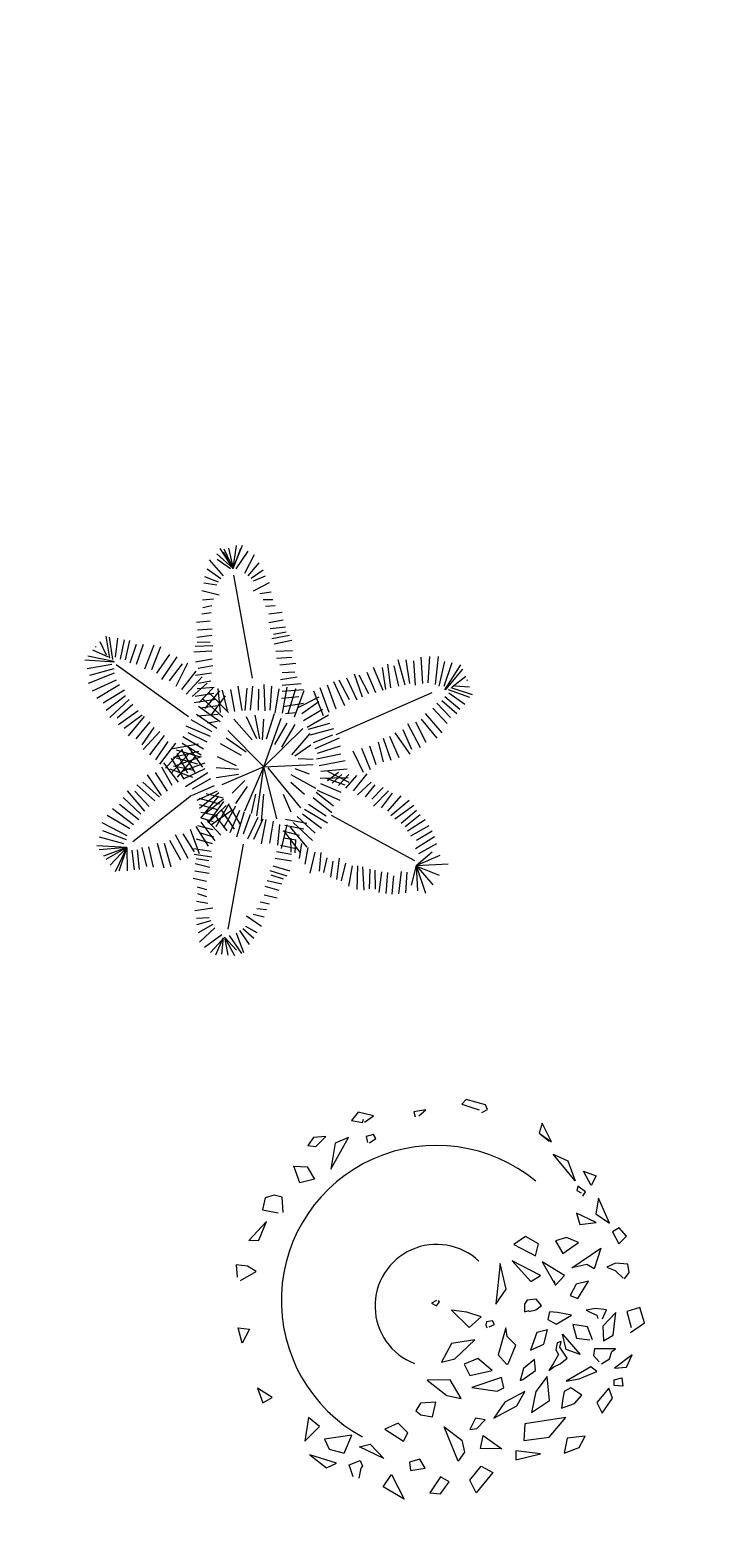
# Model space of a CAD drawing. Units: inches. Extents: x 8049 to 8459, y 820 to 1350.
# Tile 12 of 25: x 8157 to 8170, y 877 to 906. Entities that reach past the tile are written whole.
import ezdxf

# ---------------------------------------------------------------- set-up
doc = ezdxf.new("R2010")
doc.units = ezdxf.units.IN
doc.header["$MEASUREMENT"] = 0
doc.layers.add('A-ANNO-DIMS', color=2, linetype='Continuous', lineweight=18)
doc.layers.add('zelen', color=69, linetype='Continuous', lineweight=13)
doc.styles.get("Standard").update_dxf_attribs({"font": 'arial.ttf'})
doc.dimstyles.get("Standard").update_dxf_attribs({"dimtxt": 0.18, "dimasz": 0.18, "dimexe": 0.18, "dimexo": 0.0625, "dimgap": 0.09, "dimtad": 0, "dimtih": 1, "dimtoh": 1, "dimdec": 4, "dimzin": 0, "dimdsep": 46, "dimtxsty": 'Standard', "dimcen": 0.09, "dimadec": 0, "dimazin": 0, "dimtfac": 1, "dimtdec": 4, "dimtofl": 0, "dimtmove": 0, "dimatfit": 3, "dimfxl": 1, "dimtolj": 1, "dimtzin": 0, "dimarcsym": 0})

# ---------------------------------------------------------------- blocks, each defined once
blk = doc.blocks.new('z_86')
for p, q in [((-83.5, 478), (-122.3, 513.6)), ((-83.5, 478), (-114.5, 526.5)), ((-83.5, 478), (-106.5, 517.8)), ((-105.6, 525.2), (-83.5, 478)), ((-94.4, 527.5), (-83.5, 478)), ((-83.5, 478), (-61.2, 534.1)), ((-83.5, 478), (-75.1, 533.5)), ((-83.5, 478), (-65.1, 526.2)), ((-76.2, 477.3), (-47.6, 520.2)), ((-55.2, 467.1), (-32.4, 512)), ((-112.8, 453.1), (-146, 476.4)), ((-106.9, 460.9), (-139.8, 499)), ((-89.5, 477.3), (-121.9, 499.8)), ((-47.6, 461), (-21, 491.6)), ((-40, 454.9), (-11.4, 475.3)), ((-122.8, 438), (-153.5, 443.1)), ((-118.8, 445.3), (-151.4, 458.3)), ((-36.9, 215.2), (-81.5, 462)), ((-34.3, 448.8), (-5.7, 461)), ((-34.3, 424.3), (3.8, 444.7)), ((-117, 414.2), (-158.9, 425)), ((-130.3, 404.7), (-157.2, 402.3)), ((-19.1, 418.2), (7.6, 422.3)), ((-11.4, 403.9), (11.4, 403.9)), ((-135.9, 371.8), (-158.6, 368.3)), ((-134.3, 389), (-156.5, 383.5)), ((-5.7, 387.6), (17.1, 389.6)), ((1.9, 369.2), (34.3, 373.3)), ((-138.9, 352.1), (-171.3, 348.3)), ((-134, 332.3), (-168.8, 330.1)), ((1.9, 348.8), (36.2, 354.9)), ((5.7, 334.5), (41.9, 338.6)), ((13.3, 320.3), (43.8, 326.4)), ((-412.2, 291.3), (-413.8, 289.4)), ((-387.3, 269.9), (-402.1, 302.2)), ((-379.4, 263.2), (-388.4, 316.1)), ((-371.9, 259.8), (-379.8, 313.8)), ((-365.6, 265.3), (-360, 311.4)), ((-353.9, 260.7), (-343.8, 307)), ((-341.4, 258.8), (-331.3, 305.1)), ((-330.6, 251.5), (-315.1, 296.4)), ((-315.3, 248.9), (-298.9, 296.4)), ((-295.6, 237.8), (-272.9, 295.1)), ((-278.5, 236), (-256.7, 290.7)), ((-132.2, 292.8), (-174.8, 290.8)), ((-134.3, 317.5), (-170.4, 312.8)), ((-138.3, 301.8), (-169.4, 300.5)), ((9.5, 310), (51.4, 318.2)), ((15.2, 297.8), (57.1, 306)), ((-368.1, 253.4), (-438.9, 258.6)), ((-370, 255.1), (-431.7, 268)), ((-382.4, 265.8), (-420.1, 282.2)), ((-266.9, 227.1), (-235.2, 271.9)), ((-254.3, 212.2), (-218.1, 265.9)), ((-220.3, 195.8), (-192.1, 251.6)), ((-134.8, 279.6), (-177.4, 277.5)), ((-134.1, 260.9), (-173.4, 253.3)), ((19, 279.5), (59, 281.5)), ((20.9, 263.1), (57.1, 265.2)), ((329.4, 197.9), (312.2, 259.1)), ((340.8, 201.9), (331.3, 259.1)), ((354.1, 197.9), (350.3, 257)), ((371.3, 201.9), (367.5, 265.2)), ((384.6, 204), (388.4, 267.2)), ((401.7, 199.9), (409.4, 267.2)), ((411.2, 195.8), (424.6, 255)), ((422.7, 195.8), (441.7, 252.9)), ((-374.7, 247.6), (-434, 237.7)), ((-368.5, 227.2), (-431.5, 202.4)), ((-369.3, 237.5), (-427.8, 221.6)), ((-190.5, 122.3), (-363.9, 247)), ((-236.4, 208.8), (-204.7, 249.3)), ((-206.8, 187.8), (-172.4, 231.9)), ((-196.1, 176.3), (-158.1, 217.9)), ((-135.5, 226.9), (-173.5, 221.8)), ((-132, 244.6), (-167.7, 237.9)), ((28.5, 246.8), (66.6, 250.9)), ((30.5, 212.1), (70.4, 218.3)), ((34.3, 228.4), (64.7, 230.5)), ((188.5, 216.2), (213.2, 163.2)), ((226.6, 169.3), (207.5, 224.4)), ((241.8, 177.5), (218.9, 222.4)), ((258.9, 179.5), (238, 228.4)), ((276.1, 185.6), (253.2, 240.7)), ((274.2, 240.7), (281.8, 187.7)), ((295.1, 191.7), (287.5, 248.9)), ((314.1, 195.8), (302.7, 244.8)), ((424.7, 187.2), (462.5, 247.4)), ((427.1, 188.2), (467.4, 236.7)), ((442.4, 194.2), (474.5, 219.7)), ((-364.1, 210.1), (-421.7, 183.9)), ((-356, 199.3), (-410.1, 166.3)), ((-344.4, 186.1), (-394.9, 155)), ((-181.7, 171), (-145.6, 203)), ((-129.1, 192.8), (-169.4, 189.2)), ((-136.7, 207.7), (-166.7, 202.4)), ((-164.7, 156.3), (-132.2, 190.7)), ((-150.4, 142.3), (-115.1, 184.7)), ((-94.3, 132.6), (-142, 180.7)), ((-113.5, 132.6), (-119.3, 190.6)), ((-96.8, 137.1), (-108.7, 186)), ((-79.7, 135.1), (-88.7, 187.5)), ((-61.5, 137.1), (-71, 196)), ((-50.7, 191.1), (-55.5, 137.7)), ((-41.6, 138.6), (-35.8, 196)), ((-22.2, 138.2), (-21.9, 188.5)), ((-6.8, 136.7), (-9.4, 200.2)), ((5.2, 138), (9.1, 195.8)), ((17.2, 130.9), (27.2, 189.4)), ((34.3, 197.9), (80, 201.9)), ((34.3, 183.6), (85.7, 187.7)), ((34.8, 130.9), (45.8, 193.4)), ((48.3, 129.9), (66.6, 190.5)), ((64, 121.9), (87, 185.6)), ((133.3, 124.4), (110.4, 183.6)), ((146.6, 132.6), (125.6, 191.7)), ((163.7, 140.7), (142.8, 197.9)), ((184.7, 148.9), (158, 206)), ((163.8, 79.8), (394.1, 180.6)), ((196.1, 163.2), (171.3, 210.1)), ((432.2, 187.7), (483.6, 169.3)), ((438.7, 192.7), (489.7, 175.9)), ((448.3, 196.5), (483.8, 194.5)), ((478.9, 208.5), (478, 210.8)), ((-341.8, 172.4), (-387.8, 137.2)), ((-332.8, 164.2), (-378.9, 120.4)), ((-323.9, 151.7), (-361.8, 118.7)), ((-125.9, 164.1), (-176.8, 155.8)), ((-129.4, 178), (-174.7, 171)), ((-114.9, 110.1), (-166.7, 146.7)), ((-120.2, 148.7), (-161.8, 142.7)), ((-108.2, 121.8), (-155.1, 164.3)), ((-135.2, 126.7), (-101.7, 172.4)), ((32.3, 167.2), (74.2, 171.3)), ((36.2, 146.9), (85.7, 155)), ((70.9, 144), (122.8, 170.4)), ((81, 130), (122.3, 158.8)), ((405.5, 155), (437.9, 120.3)), ((417, 161.2), (453.2, 130.5)), ((424.6, 171.3), (460.8, 140.7)), ((434.1, 179.5), (472.2, 153)), ((-311.3, 136.8), (-358.3, 103.3)), ((-344.8, 95.3), (-301.5, 126.9)), ((-297, 122.8), (-335, 76.8)), ((-283.6, 110.5), (-317, 69.1)), ((-134, 86.3), (-184.5, 114.7)), ((-122.5, 94.2), (-171, 128.2)), ((-119, 128), (-169, 124.1)), ((-120.6, 110.8), (-145.2, 106.9)), ((-38.1, 67.3), (-81.9, 116.3)), ((-26.7, 69.3), (-51.4, 122.4)), ((-19.1, 69.3), (-30.5, 126.5)), ((-13.3, 67.3), (-9.5, 116.3)), ((-9.5, 2), (31.9, 119.3)), ((-3.8, 69.5), (16, 129.9)), ((41.9, 130.5), (66.6, 132.6)), ((85.4, 113.4), (131, 140.8)), ((93.8, 97.2), (145.2, 127.4)), ((354.1, 110.1), (378.9, 61.2)), ((367.5, 116.3), (405.5, 71.4)), ((377, 130.5), (417, 83.6)), ((396, 142.8), (430.3, 106.1)), ((-273.8, 96.3), (-302.7, 55.1)), ((-259.4, 86.7), (-299.2, 44.1)), ((-283.1, 31.1), (-247.8, 77.8)), ((-154.7, 44.3), (-204, 74.1)), ((-138, 74.9), (-196.4, 99.8)), ((-145.9, 61.7), (-191.3, 83.5)), ((-9.5, 2), (-96.2, 89.6)), ((-9.5, 2), (83.8, 94.2)), ((16.7, 55.7), (46.5, 106.9)), ((33.2, 49.6), (65.3, 104.2)), ((57.4, 30.9), (101.2, 82.5)), ((148.1, 106.6), (96.6, 91.8)), ((102.5, 79.2), (158, 94.6)), ((109.1, 60.9), (156.1, 78.9)), ((291.3, 75.5), (314.1, 24.4)), ((304.6, 83.6), (340.8, 32.6)), ((323.7, 91.8), (344.6, 44.9)), ((335.1, 106.1), (365.5, 48.9)), ((-239.8, 62.7), (-269.6, 18.8)), ((-221.8, 59.2), (-259.8, 8.9)), ((-204.8, 44.6), (-245.5, -0.7)), ((-166.3, 56.4), (-233.1, 45)), ((-165.5, 38.8), (-227.2, 24.8)), ((-161.8, 25.7), (-219.1, 42.3)), ((-174.2, -11.2), (-206.8, 42.8)), ((-206, 58.7), (-159.8, 31.4)), ((-155.8, 1.7), (-191.5, 50.9)), ((-63.5, 29.2), (-114, 57.6)), ((-52, 37.1), (-100.5, 71.1)), ((64.7, 28.6), (102.8, 55.1)), ((113.3, 46.1), (171.5, 71.5)), ((118.9, 35.3), (174.1, 52.6)), ((203.7, 40.8), (228.5, -10.2)), ((224.7, 46.9), (245.6, -4.1)), ((243.7, 53), (258.9, 8.1)), ((264.6, 61.2), (276.1, 14.3)), ((276.1, 71.4), (295.1, 18.4)), ((-229.7, -42.7), (-254.3, 1.3)), ((-214.5, -34.6), (-249.6, 11.9)), ((-232.2, 23.2), (-202, -27)), ((-189.6, 33.2), (-232, -13)), ((-176.9, -6.2), (-226.2, 4.1)), ((-159.8, 26.6), (-219.4, 5.3)), ((-167.8, 8.5), (-219.1, 22.8)), ((-176.1, 25.3), (-217.7, -22.6)), ((-192.4, -12.7), (-217.6, 34)), ((-151.1, 11.3), (-206.8, -8.9)), ((-70.4, -4.1), (-123.8, 0)), ((-75.4, 4.6), (-120.8, 26.4)), ((-9.5, 2), (-110.4, -40.8)), ((-55.6, -103.4), (-9.5, 2)), ((-26.9, -115.3), (-9.5, 2)), ((-9.5, 2), (108.5, 8.1)), ((-9.5, 0), (20.9, -122.4)), ((0, 0), (78, -95.9)), ((72.4, 22.4), (108.5, 20.4)), ((116.7, 21.6), (174.7, 33.4)), ((123, 5.1), (185.2, 17.6)), ((-300.3, -34.4), (-260.5, -70.2)), ((-255.6, -66.7), (-288.6, -17)), ((-241, -55.8), (-270, -11.1)), ((-180.1, -23.2), (-234.9, -3.5)), ((-151.3, -2.6), (-203.4, -27.7)), ((-144.2, -12.5), (-198.1, -46)), ((-137.9, -26.5), (-181.8, -51.2)), ((-70.4, -16.3), (-123.8, -24.5)), ((-55.2, -30.6), (-85.7, -61.2)), ((55.2, -16.3), (114.2, -49)), ((55.2, -34.7), (87.6, -63.3)), ((64.7, -2.1), (99, -14.3)), ((125.2, -25.3), (192.9, -23.6)), ((126.9, -7.8), (190, -2.9)), ((137.2, -24.2), (184.8, -40.9)), ((142.6, -7.8), (194.4, -34.4)), ((142.8, -30.6), (169.5, -10.2)), ((154.2, -36.8), (177.1, -16.3)), ((169.5, -42.8), (194.2, -16.3)), ((186.6, -49), (213.2, -18.4)), ((205.6, -55.1), (238, -14.3)), ((215.1, -65.3), (247.5, -34.7)), ((-305.2, -111.3), (-347.4, -71.6)), ((-295.5, -104.1), (-336.7, -55.7)), ((-183, -66.2), (-324.2, -177.7)), ((-285.3, -92.6), (-319.6, -55.8)), ((-271.3, -79), (-314.5, -40.9)), ((-128.7, -43.7), (-181.4, -66.9)), ((-169.9, -77.5), (-121.1, -55.3)), ((-117.5, -60.2), (-164, -97.6)), ((-118.6, -68.3), (-161.5, -120.7)), ((-107.6, -72.7), (-148.4, -62.3)), ((-49.5, -44.9), (-78.1, -85.7)), ((-39.1, -109.5), (-28.6, -63.3)), ((-15, -128.2), (-9.5, -63.3)), ((36.2, -63.3), (55.2, -106.1)), ((108.5, -71.4), (153.5, -107.4)), ((157.5, -92.3), (115.4, -59.2)), ((118.1, -53.8), (172.7, -77.8)), ((126.3, -37.5), (175.2, -58.4)), ((234.2, -69.4), (257, -40.8)), ((249.4, -75.5), (276.1, -47)), ((253.2, -91.8), (289.4, -55.1)), ((272.2, -95.9), (298.9, -61.2)), ((287.5, -104.1), (319.9, -67.3)), ((-322.2, -136.6), (-372.6, -98.2)), ((-309.3, -124.6), (-356.3, -88.5)), ((-115, -87.4), (-164.7, -73.8)), ((-119.8, -100.8), (-164.2, -89.1)), ((-106.9, -75), (-148, -108.8)), ((-106.4, -81), (-143.8, -132.1)), ((-100.1, -90.9), (-136.8, -125.4)), ((-88, -103.2), (-135.6, -136.9)), ((-94.1, -86.5), (-125.1, -141.7)), ((-111.8, -101.2), (-81.1, -147)), ((-77.5, -92.3), (-106.3, -144.1)), ((-95, -87.2), (-66.5, -136.2)), ((-68.5, -102.9), (-91.4, -156.1)), ((-56.7, -105.7), (-75.4, -166.5)), ((88, -99.5), (142.7, -131.9)), ((97.6, -87.5), (139.7, -115)), ((295.1, -114.2), (338.9, -77.5)), ((304.6, -122.4), (350.3, -89.8)), ((319.9, -132.6), (356.1, -102)), ((-337.4, -163), (-397.6, -131.9)), ((-331.3, -146.5), (-385.9, -114.5)), ((-172.6, -140.6), (-143, -188)), ((-131.1, -148.8), (-168.3, -139.7)), ((-121.1, -115.5), (-160.8, -107.7)), ((-160.7, -130.3), (-127.3, -175.6)), ((-130.2, -129.6), (-159.6, -121.2)), ((-145.9, -126.4), (-113.3, -162.1)), ((-127.4, -113.6), (-98.7, -151.2)), ((-42.8, -112.2), (-59.7, -159.6)), ((-24.5, -119.1), (-49, -171.2)), ((-33.4, -171.6), (-11.1, -122.9)), ((-5.2, -124.2), (-15.8, -182.9)), ((12.5, -128.4), (3.6, -180.9)), ((28, -135.9), (23, -186.1)), ((45.2, -137.3), (31.5, -193.9)), ((40.8, -137.7), (85.8, -146.5)), ((42.3, -123.5), (93, -132.9)), ((52.3, -142.1), (93.3, -190.4)), ((60.6, -131.4), (107, -174.5)), ((70.1, -116.6), (113.7, -156.7)), ((82.6, -110.3), (128.9, -145)), ((151.4, -114), (352, -222.7)), ((329.4, -140.8), (365.5, -112.2)), ((335.1, -151), (377, -124.4)), ((342.7, -163.2), (386.5, -138.7)), ((-345.7, -182.7), (-403.8, -166.7)), ((-339.4, -173.2), (-395.9, -151.3)), ((-236.4, -173.5), (-209.5, -221.3)), ((-222.4, -160), (-191.9, -217.1)), ((-204.2, -158.4), (-176.9, -202)), ((-186.8, -147.2), (-164.6, -205.6)), ((-133.2, -182.8), (-171.5, -171.1)), ((-129.5, -166.7), (-164.2, -156.4)), ((35.5, -151.5), (74.7, -161.8)), ((37.1, -150.9), (78.1, -204.9)), ((37.6, -168.1), (67.7, -173.3)), ((54.3, -168.6), (55, -202.2)), ((66.2, -173.7), (64.5, -204.3)), ((354.1, -193.8), (399.8, -165.3)), ((356.1, -173.4), (394.1, -151)), ((-338.1, -191.4), (-410.8, -187.1)), ((-338.1, -191.4), (-404.6, -197.1)), ((-338.1, -191.4), (-394.5, -212.5)), ((-338.1, -191.4), (-389, -220.3)), ((-338.1, -191.4), (-378.7, -234.2)), ((-338.1, -191.4), (-366.5, -249.5)), ((-338.1, -191.4), (-357.7, -248.1)), ((-338.1, -191.4), (-337.7, -247.7)), ((-326.5, -197.9), (-321.2, -245)), ((-313.8, -197.3), (-308.5, -244.4)), ((-302.3, -191.2), (-291.5, -237.4)), ((-286.8, -190.1), (-275.4, -239)), ((-266.1, -181.1), (-249.4, -240.5)), ((-248.9, -181.2), (-232.8, -237.8)), ((-135.9, -201.3), (-178, -194.7)), ((-134.7, -214.7), (-176.8, -208.2)), ((-59.2, -183), (-96.3, -387.3)), ((20.7, -201.2), (56.5, -207.1)), ((30, -185.8), (67.5, -193.9)), ((80.5, -181.8), (75.2, -217.7)), ((96, -191.4), (88.7, -231.3)), ((112.6, -202.4), (100.9, -253.2)), ((126.6, -203.5), (122.8, -247.9)), ((355.4, -234.4), (394.1, -202)), ((355.4, -234.4), (413.2, -210.1)), ((361.7, -206.1), (405.5, -181.6)), ((-140.6, -253.8), (-175, -247.9)), ((-139.4, -239.1), (-174.8, -230.6)), ((-141.7, -223), (-172.4, -218.5)), ((4.5, -246.7), (45.3, -259.2)), ((11.4, -235.1), (52.2, -247.6)), ((17.1, -217.3), (56.7, -223.5)), ((141.6, -215.8), (133.6, -251.5)), ((155.9, -223.9), (150.3, -262.6)), ((171, -216.7), (164.9, -267.9)), ((186.1, -229), (175.7, -271.5)), ((202, -235.8), (193.5, -284.1)), ((214.7, -235.4), (213.3, -292.5)), ((227, -237.7), (230.1, -293.8)), ((244.5, -243.3), (243.2, -290.7)), ((256.8, -245.6), (257.1, -291.7)), ((272.4, -249.9), (266.2, -299.1)), ((319.3, -248.8), (312.9, -302.4)), ((333.6, -250.5), (330.1, -300.5)), ((355.4, -234.4), (343.7, -281.5)), ((354.7, -235.1), (410.6, -257.7)), ((355.4, -234.4), (432.2, -230.9)), ((355.4, -234.4), (359.2, -295.3)), ((355.4, -234.4), (378.3, -301.1)), ((355.4, -234.4), (395.7, -281.2)), ((-147.6, -273), (-179.4, -265.8)), ((-146.7, -292.8), (-168.8, -287)), ((-7.2, -284.4), (26.3, -294.1)), ((-1.9, -270.6), (33.7, -278.5)), ((7.2, -257.2), (36.8, -266.5)), ((286.7, -251.6), (283.2, -301.6)), ((301.6, -259.3), (297.6, -303.3)), ((-144.5, -326.2), (-171, -321)), ((-146.8, -310.2), (-168.3, -302.4)), ((-18.8, -322.2), (3.7, -326.6)), ((-9.3, -304.7), (22.5, -312.2)), ((-132.2, -337.1), (-175, -343.3)), ((-51.1, -355.7), (-15.3, -380)), ((-35.3, -351.3), (-9.2, -358.1)), ((-26.2, -337.8), (-3.5, -340.2)), ((-140.6, -360.1), (-171.6, -361.9)), ((-137.3, -367.8), (-171.1, -377.3)), ((-132.2, -376.2), (-167.6, -395.9)), ((-127.1, -384.5), (-163.8, -418.9)), ((-68.2, -390.9), (-44.9, -424.1)), ((-59.9, -385.6), (-33.7, -408.9)), ((-53.6, -380.1), (-26.5, -395.3)), ((-110.9, -401.2), (-152.3, -431.8)), ((-110.9, -413.5), (-137.9, -443.4)), ((-124.9, -449.3), (-107.4, -408)), ((-107.4, -408), (-111.5, -447.2)), ((-104.4, -407), (-96.1, -449.6)), ((-104.4, -407), (-79.8, -451)), ((-104.4, -407), (-75.5, -437.8)), ((-92.8, -402.8), (-63.3, -445.5)), ((-76.4, -396.1), (-58.3, -443.2))]:
    blk.add_line(p, q)
blk = doc.blocks.new('z_66')
for p, q in [((83.2, 488.9), (72.7, 477.7)), ((72.7, 477.7), (96.4, 469.7)), ((129.8, 476.2), (83.2, 488.9)), ((96.4, 469.7), (114.5, 463.9)), ((134, 464.6), (129.8, 476.2)), ((-176.4, 458.5), (-191.7, 438.6)), ((-191.7, 438.6), (-165.6, 433.5)), ((-139.2, 449.4), (-176.4, 458.5)), ((-165.6, 433.5), (-163.6, 441.1)), ((-165.6, 433.5), (-165.6, 433.5)), ((-161.1, 434.6), (-139.2, 449.4)), ((-13.6, 463.6), (-42.5, 459.2)), ((-42.5, 459.2), (-39.3, 446.9)), ((-30.3, 449.4), (-13.6, 463.6)), ((114.5, 463.9), (114.5, 463.9)), ((120.4, 457.8), (134, 464.6)), ((265.2, 432.1), (258.2, 407.5)), ((287.4, 387.2), (265.2, 432.1)), ((-283.6, 397.7), (-297.2, 378.2)), ((-254, 399.9), (-283.6, 397.7)), ((-272.8, 380.7), (-254, 399.9)), ((-241.9, 321.7), (-199.1, 397.3)), ((-199.1, 397.3), (-231.4, 383.6)), ((-138.9, 404.9), (-156.9, 400.2)), ((-156.9, 400.2), (-153.8, 385.4)), ((-133.3, 394.8), (-138.9, 404.9)), ((258.2, 407.5), (287.4, 387.2)), ((258.2, 407.5), (281.9, 388.6)), ((-297.2, 378.2), (-277.7, 376)), ((-277.7, 376), (-272.8, 380.7)), ((-231.4, 383.6), (-241.9, 321.7)), ((-148.6, 384.7), (-133.3, 394.8)), ((281.9, 388.6), (281.9, 388.6)), ((-330.3, 328.9), (-298.6, 327.1)), ((-316, 288.8), (-330.3, 328.9)), ((-298.6, 327.1), (-280.8, 297.1)), ((344.2, 293.1), (292, 357.2)), ((292, 357.2), (326.8, 341.2)), ((326.8, 341.2), (344.2, 293.1)), ((-280.8, 297.1), (-316, 288.8)), ((383.1, 281.9), (364.4, 316.3)), ((364.4, 316.3), (394.6, 305.1)), ((394.6, 305.1), (383.1, 281.9)), ((-399.2, 252.6), (-405.8, 224)), ((-377.9, 259.1), (-399.2, 252.6)), ((-358.4, 254), (-377.9, 259.1)), ((-356, 217.5), (-358.4, 254)), ((350.8, 280.8), (348.7, 270.3)), ((348.7, 270.3), (358.8, 264.5)), ((369.2, 266.7), (350.8, 280.8)), ((358.8, 264.5), (358.8, 264.5)), ((363.3, 256.6), (369.2, 266.7)), ((400.9, 251.9), (393.9, 214.6)), ((426.6, 192.2), (400.9, 251.9)), ((-405.8, 224), (-368.2, 216.4)), ((-368.2, 216.4), (-368.2, 216.4)), ((348, 215.7), (356, 188.9)), ((395.3, 193.2), (348, 215.7)), ((-396.4, 196.1), (-438.1, 150.2)), ((-414.8, 150.9), (-396.4, 196.1)), ((356, 188.9), (395.3, 193.2)), ((393.9, 214.6), (426.6, 192.2)), ((450, 180.6), (434.3, 171.2)), ((467.7, 160.3), (450, 180.6)), ((-438.1, 150.2), (-414.8, 150.9)), ((225.2, 159.9), (197, 140.8)), ((256.8, 142.6), (225.2, 159.9)), ((323.6, 157.8), (297.5, 149.8)), ((297.5, 149.8), (314.6, 119.4)), ((314.6, 119.4), (352.9, 145.5)), ((352.9, 145.5), (323.6, 157.8)), ((434.3, 171.2), (449.6, 142.6)), ((449.6, 142.6), (467.7, 160.3)), ((197, 140.8), (249.5, 113.6)), ((249.5, 113.6), (256.8, 142.6)), ((336.9, 84.3), (405.8, 131.7)), ((405.8, 131.7), (389.8, 82.1)), ((-468.4, 91.6), (-466.3, 62.6)), ((-441.6, 89), (-468.4, 91.6)), ((-458.3, 53.9), (-421.1, 76)), ((-421.1, 76), (-441.6, 89)), ((164.3, 94.8), (154.2, -2.2)), ((178.9, 33.3), (164.3, 94.8)), ((193.1, 101.3), (238, 52.1)), ((261.7, 66.6), (193.1, 101.3)), ((265.2, 98.8), (297.2, 42.7)), ((318.8, 66.2), (265.2, 98.8)), ((372.7, 93), (336.9, 84.3)), ((389.8, 82.1), (372.7, 93)), ((441.6, 95.9), (420.7, 86.5)), ((420.7, 86.5), (440.2, 78.5)), ((440.2, 78.5), (459.7, 59.7)), ((470.5, 93.7), (441.6, 95.9)), ((463.2, 57.9), (474, 73.5)), ((474, 73.5), (470.5, 93.7)), ((-466.3, 62.6), (-466.3, 62.6)), ((238, 52.1), (261.7, 66.6)), ((297.2, 42.7), (294.1, 53.6)), ((297.2, 42.7), (318.8, 66.2)), ((347.3, 45.2), (332.7, 18.1)), ((376.9, 52.5), (347.3, 45.2)), ((350.8, 10.9), (376.9, 52.5)), ((459.7, 59.7), (459.7, 59.7)), ((11.8, 6.2), (0, 0)), ((0, 0), (12.2, -6.9)), ((12.2, -6.9), (19.1, 2.9)), ((19.1, 2.9), (15.7, 5.8)), ((154.2, -2.2), (178.9, 33.3)), ((229, 7.2), (223.1, -2.5)), ((250.6, 9.8), (229, 7.2)), ((263.4, -5.4), (250.6, 9.8)), ((332.7, 18.1), (350.8, 10.9)), ((84.6, -21.7), (48, -17)), ((48, -17), (90.1, -58.3)), ((119.4, -32.9), (84.6, -21.7)), ((90.1, -58.3), (119.4, -32.9)), ((223.1, -2.5), (222.7, -20.6)), ((222.7, -20.6), (234.2, -18.1)), ((233.2, -19.9), (249.9, -15.9)), ((234.2, -18.1), (234.2, -18.1)), ((249.9, -15.9), (263.4, -5.4)), ((282.9, -21.3), (279.1, -39.1)), ((302.1, -22.8), (282.9, -21.3)), ((298.6, -50.3), (335.8, -28.6)), ((335.8, -28.6), (302.1, -22.8)), ((393.6, -13), (371, -17)), ((371, -17), (383.5, -23.5)), ((383.5, -23.5), (396.7, -28.9)), ((420, -15.9), (393.6, -13)), ((396.7, -28.9), (398.5, -35.5)), ((398.5, -35.5), (399.5, -35.8)), ((410.3, -38), (420, -15.9)), ((442, -22.4), (411.3, -55.4)), ((436, -77.1), (442, -22.4)), ((499.7, -10.9), (468.8, -19.9)), ((468.8, -19.9), (478.8, -58.6)), ((510.9, -47), (499.7, -10.9)), ((-464.2, -59.3), (-436.4, -62.6)), ((-454.5, -96.3), (-464.2, -59.3)), ((-436.4, -62.6), (-454.5, -96.3)), ((131.9, -44.9), (130.2, -52.5)), ((130.2, -52.5), (132.9, -59.3)), ((146.5, -42.3), (131.9, -44.9)), ((138.2, -56.8), (151, -51)), ((151, -51), (146.5, -42.3)), ((177.8, -59), (160.1, -123.8)), ((181, -80.3), (177.8, -59)), ((252.6, -70.9), (237.7, -112.9)), ((278.4, -64), (252.6, -70.9)), ((269.7, -98.4), (278.4, -64)), ((279.1, -39.1), (298.6, -50.3)), ((339, -51), (347.7, -84.3)), ((374.1, -56.8), (339, -51)), ((386.3, -87.9), (374.1, -56.8)), ((411.3, -55.4), (412.7, -90.8)), ((477.5, -70.2), (510.9, -47)), ((478.8, -58.6), (478.8, -58.6)), ((47.7, -96.6), (24, -141.9)), ((104.1, -87.9), (47.7, -96.6)), ((56, -133.9), (104.1, -87.9)), ((202.2, -100.6), (181, -80.3)), ((183.7, -145.5), (202.2, -100.6)), ((237.7, -112.9), (269.7, -98.4)), ((301.7, -95.5), (297.9, -112.2)), ((310.8, -91.9), (301.7, -95.5)), ((307.6, -106), (310.8, -91.9)), ((325.4, -132.4), (307.6, -106)), ((314.2, -74.2), (356.7, -123)), ((323.3, -111.1), (314.2, -74.2)), ((347.7, -84.3), (379.7, -88.3)), ((379.7, -88.3), (379.7, -88.3)), ((412.7, -90.8), (436, -77.1)), ((24, -141.9), (56, -133.9)), ((111.4, -132.8), (78.3, -146.2)), ((145.1, -162.1), (111.4, -132.8)), ((160.1, -123.8), (179.6, -146.6)), ((247.1, -135.7), (220.6, -157)), ((249.2, -162.1), (247.1, -135.7)), ((304.5, -123), (291.6, -145.8)), ((297.9, -112.2), (304.5, -123)), ((308.3, -145.8), (325.4, -132.4)), ((356.7, -123), (323.3, -111.1)), ((356.7, -123), (356.7, -123)), ((356.7, -123), (356.7, -123)), ((391.2, -110), (388.4, -125.6)), ((388.4, -125.6), (402.3, -140.8)), ((391.2, -110), (393.2, -108.6)), ((441.3, -110), (391.2, -110)), ((402.3, -140.8), (402.3, -140.8)), ((407.9, -145.5), (427, -133.5)), ((427, -133.5), (432.9, -115.8)), ((432.9, -115.8), (441.3, -110)), ((480.9, -124.5), (439.2, -156)), ((467.7, -153.4), (480.9, -124.5)), ((78.3, -146.2), (92.2, -174.1)), ((92.2, -174.1), (145.1, -162.1)), ((168.1, -178.4), (96.7, -202.6)), ((173, -203.4), (168.1, -178.4)), ((179.6, -146.6), (183.7, -145.5)), ((220.6, -157), (212.6, -186)), ((219.2, -183.5), (249.2, -162.1)), ((277.4, -176.2), (250.2, -212.4)), ((283.3, -233.8), (277.4, -176.2)), ((291.6, -145.8), (281.2, -161.8)), ((281.2, -161.8), (293, -152.7)), ((293, -152.7), (308.3, -145.8)), ((382.5, -152.7), (323.3, -187.4)), ((353.9, -182), (396.7, -164.3)), ((396.7, -164.3), (382.5, -152.7)), ((438.5, -183.8), (456.2, -179.1)), ((439.2, -156), (467.7, -153.4)), ((456.2, -179.1), (458.7, -199)), ((-417.9, -204.1), (-405.1, -239.6)), ((-382.8, -226.5), (-417.9, -204.1)), ((44.5, -184.2), (-10.8, -184.9)), ((-10.8, -184.9), (36.9, -222.2)), ((71, -229.1), (44.5, -184.2)), ((96.7, -202.6), (157.6, -211.3)), ((157.6, -211.3), (173, -203.4)), ((223.8, -212.4), (175.4, -237.7)), ((204.3, -246.8), (223.8, -212.4)), ((212.6, -186), (219.2, -183.5)), ((250.2, -212.4), (240.1, -262.4)), ((318.4, -212.1), (314.6, -228.7)), ((334.1, -203.7), (318.4, -212.1)), ((323.3, -187.4), (353.9, -182)), ((360.2, -221.1), (334.1, -203.7)), ((425.3, -204.5), (396.7, -238.5)), ((434.3, -228), (425.3, -204.5)), ((438.5, -197.6), (438.5, -183.8)), ((458.7, -199), (438.5, -197.6)), ((-405.1, -239.6), (-382.8, -226.5)), ((-26.4, -240.3), (-37.6, -258.4)), ((10.1, -237.7), (-26.4, -240.3)), ((2.4, -273.2), (10.1, -237.7)), ((36.9, -222.2), (71, -229.1)), ((175.4, -237.7), (149.6, -276.1)), ((149.6, -276.1), (204.3, -246.8)), ((240.1, -262.4), (283.3, -233.8)), ((314.6, -228.7), (311.8, -252.6)), ((311.8, -252.6), (320.5, -249.3)), ((320.5, -249.3), (342.8, -241.4)), ((342.8, -241.4), (360.2, -221.1)), ((396.7, -238.5), (409.2, -264.2)), ((409.2, -264.2), (434.3, -228)), ((-295.1, -275), (-304.2, -331.5)), ((-269, -296), (-295.1, -275)), ((-37.6, -258.4), (-25.8, -268.5)), ((-25.8, -268.5), (2.4, -273.2)), ((-25.8, -268.5), (-25.8, -268.5)), ((-25.8, -268.5), (-25.8, -268.5)), ((105.1, -276.1), (91.9, -303.6)), ((128.8, -280.4), (105.1, -276.1)), ((108.6, -301.4), (128.8, -280.4)), ((322.2, -275), (223.8, -290.2)), ((282.2, -321.7), (322.2, -275)), ((-304.2, -331.5), (-269, -296)), ((-191.1, -317.4), (-256.8, -326.4)), ((-209.8, -360.4), (-191.1, -317.4)), ((-80, -288), (-112.4, -302.5)), ((-112.4, -302.5), (-67.5, -331.8)), ((-56.7, -311.6), (-80, -288)), ((-67.5, -331.8), (-56.7, -311.6)), ((30.6, -297.1), (72.7, -329.3)), ((64, -379.6), (30.6, -297.1)), ((91.9, -303.6), (108.6, -301.4)), ((117.3, -348.8), (124.2, -317.7)), ((124.2, -317.7), (168.8, -349.9)), ((223.8, -290.2), (221.3, -330)), ((221.3, -330), (282.2, -321.7)), ((368.9, -319.2), (325.7, -323.9)), ((354.3, -346.3), (368.9, -319.2)), ((-256.8, -326.4), (-245.7, -350.3)), ((-245.7, -350.3), (-209.8, -360.4)), ((-172.6, -344.9), (-146.9, -338.7)), ((-114.8, -372.7), (-172.6, -344.9)), ((-146.9, -338.7), (-114.8, -372.7)), ((79.3, -357.9), (64, -379.6)), ((72.7, -329.3), (79.3, -357.9)), ((168.8, -349.9), (117.3, -348.8)), ((201.8, -355), (202.2, -376.3)), ((261, -362.2), (201.8, -355)), ((325.7, -323.9), (318.4, -360.1)), ((318.4, -360.1), (354.3, -346.3)), ((-292, -364.4), (-252, -395.5)), ((-228.3, -383.9), (-292, -364.4)), ((-252, -395.5), (-228.3, -383.9)), ((-197.3, -388.3), (-171.2, -377.8)), ((-188.3, -416.9), (-197.3, -388.3)), ((-171.2, -377.8), (-166, -391.5)), ((-166, -391.5), (-169.5, -396.6)), ((-27.8, -374.5), (-52.9, -381.8)), ((-52.9, -381.8), (-50.8, -402)), ((-15.3, -396.2), (-27.8, -374.5)), ((91.9, -424.8), (119, -391.5)), ((119, -391.5), (146.9, -406.4)), ((202.2, -376.3), (261, -362.2)), ((-169.5, -396.6), (-174.7, -420.5)), ((-174.7, -420.5), (-174.7, -420.5)), ((-116.2, -441.1), (-96.4, -411.8)), ((-96.4, -411.8), (-65.8, -470.8)), ((-50.8, -402), (-15.3, -396.2)), ((21.6, -417.2), (-4.5, -455.6)), ((42.1, -428.8), (21.6, -417.2)), ((21.6, -458.1), (42.1, -428.8)), ((106.8, -455.6), (91.9, -424.8)), ((146.9, -406.4), (106.8, -455.6)), ((-65.8, -470.8), (-116.2, -441.1)), ((-4.5, -455.6), (21.6, -458.1))]:
    blk.add_line(p, q)
for centre, radius, start, end in [((11.8, 6.2), 372.3, 50.2118, 241.5185), ((12.2, -6.9), 147.8, 46.7611, 248.9067)]:
    blk.add_arc(centre, radius, start, end)
blk = doc.blocks.new('*D58')
at = {"layer": 'A-ANNO-DIMS', "color": 0, "lineweight": -2, "transparency": 16777216}
for p, q in [((8139.397, 1162.808), (8139.397, 820.091)), ((8175.397, 1162.808), (8175.397, 820.091)), ((8139.577, 820.271), (8157.179, 820.271)), ((8175.217, 820.271), (8157.616, 820.271))]:
    blk.add_line(p, q, dxfattribs=at)
at = {"layer": 'A-ANNO-DIMS', "color": 0, "transparency": 16777216}
for points in [[(8139.577, 820.301), (8139.577, 820.241), (8139.397, 820.271)], [(8175.217, 820.301), (8175.217, 820.241), (8175.397, 820.271)]]:
    blk.add_solid(points, dxfattribs=at)
at = {"layer": 'Defpoints', "color": 0, "transparency": 16777216}
for p in [(8139.397, 1162.871), (8175.397, 1162.871), (8175.397, 820.271)]:
    blk.add_point(p, dxfattribs=at)
at = {"layer": 'A-ANNO-DIMS', "color": 0, "transparency": 16777216, "insert": (8157.397, 820.271), "char_height": 0.18, "attachment_point": 5}
blk.add_mtext('\\A1;36', dxfattribs=at)
blk = doc.blocks.new('*D76')
at = {"layer": 'A-ANNO-DIMS', "color": 0, "lineweight": -2, "transparency": 16777216}
for p, q in [((8083.397, 1054.808), (8083.397, 820.091)), ((8299.397, 1054.808), (8299.397, 820.091)), ((8083.577, 820.271), (8191.107, 820.271)), ((8299.217, 820.271), (8191.688, 820.271))]:
    blk.add_line(p, q, dxfattribs=at)
at = {"layer": 'A-ANNO-DIMS', "color": 0, "transparency": 16777216}
for points in [[(8083.577, 820.301), (8083.577, 820.241), (8083.397, 820.271)], [(8299.217, 820.301), (8299.217, 820.241), (8299.397, 820.271)]]:
    blk.add_solid(points, dxfattribs=at)
at = {"layer": 'Defpoints', "color": 0, "transparency": 16777216}
for p in [(8083.397, 1054.871), (8299.397, 1054.871), (8299.397, 820.271)]:
    blk.add_point(p, dxfattribs=at)
at = {"layer": 'A-ANNO-DIMS', "color": 0, "transparency": 16777216, "insert": (8191.397, 820.271), "char_height": 0.18, "attachment_point": 5}
blk.add_mtext('\\A1;216', dxfattribs=at)

msp = doc.modelspace()

# ---------------------------------------------------------------- block references
at = {"layer": 'zelen', "xscale": 0.0082668533249786, "yscale": 0.0082668533249786, "zscale": 0.0082668533249786}
for name, p in [('z_86', (8161.3792, 891.6377)), ('z_66', (8164.6248, 881.015))]:
    msp.add_blockref(name, p, dxfattribs=at)

# ---------------------------------------------------------------- dimensions: what is measured, and where the dimension line sits
at = {"layer": 'A-ANNO-DIMS'}
for base, p1, p2, picture, middle in [((8175.3974, 820.2706), (8139.3974, 1162.8706), (8175.3974, 1162.8706), '*D58', (8157.3974, 820.2706)), ((8299.3974, 820.2706), (8083.3974, 1054.8706), (8299.3974, 1054.8706), '*D76', (8191.3974, 820.2706))]:
    dim = msp.add_linear_dim(base=base, p1=p1, p2=p2, dimstyle='Standard', override={"dimdec": 0, "dimlfac": 1, "dimrnd": 0, "dimzin": 0, "dimdsep": 46, "dimlunit": 2}, dxfattribs=at)
    dim.commit()
    dim.dimension.update_dxf_attribs({"geometry": picture, "text_midpoint": middle})

doc.saveas('drawing.dxf')
